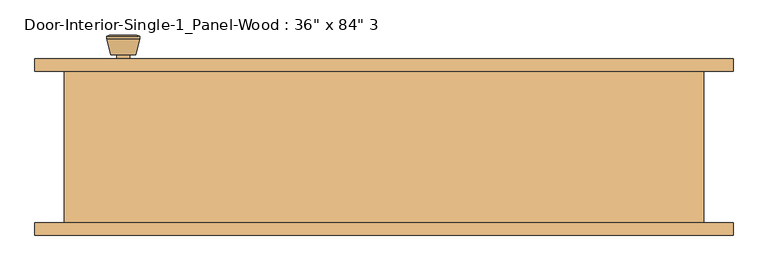
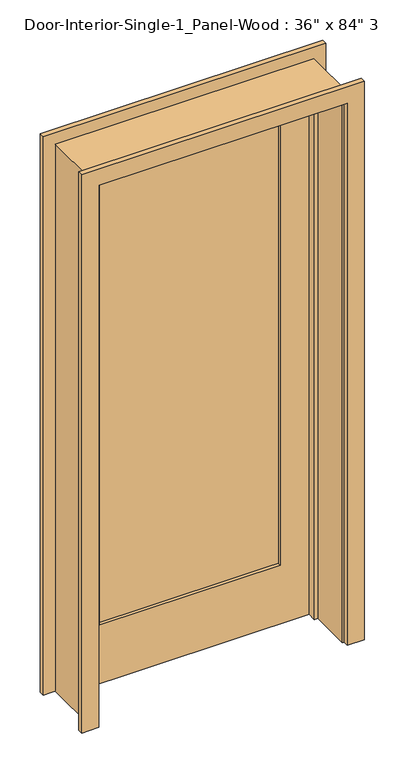
"""IFC4 building model written with IfcOpenShell, lengths in millimetres: door geometry."""

from ifc_helpers import new_model, si_unit, point, frame, frame_2d, origin, place, context, project, spatial, polyline, circle_curve, trimmed, segment, composite_curve, outline, extrude, faceted_brep, source, transform, mapped, element, save
from ifc_brep_helpers import plane_surface, cylinder_surface, revolved_surface, advanced_brep


def door_3b97b8e7(model_context):
    return source(origin(), model_context, "Body", "SolidModel", [
        advanced_brep(
        [(-393.7, 70.2, 914.4), (-383.7, 70.2, 914.4), (-403.7, 70.2, 914.4), (-373.2241324, 21.2, 914.4), (-393.7, 21.2, 914.4), (-414.1758676, 21.2, 914.4), (-368.7, 23.0278681, 914.4), (-418.7, 23.0278681, 914.4), (-368.7, 26.4915463, 914.4), (-418.7, 26.4915463, 914.4), (-375.063764, 51.2, 914.4), (-412.336236, 51.2, 914.4), (-383.7, 51.2, 914.4), (-403.7, 51.2, 914.4)],
        [
            (0, 1),
            (1, 2, circle_curve(frame((-393.7, 70.2, 914.4), z_axis=(0.0, 1.0, 0.0), x_axis=(-1.0, 0.0, 0.0)), 10.0)),
            (2, 0),
            (2, 1, circle_curve(frame((-393.7, 70.2, 914.4), z_axis=(0.0, 1.0, 0.0), x_axis=(-1.0, 0.0, 0.0)), 10.0)),
            (3, 4),
            (4, 5),
            (5, 3, circle_curve(frame((-393.7, 21.2, 914.4), z_axis=(0.0, -1.0, 0.0), x_axis=(-1.0, 0.0, 0.0)), 20.4758676)),
            (3, 5, circle_curve(frame((-393.7, 21.2, 914.4), z_axis=(0.0, -1.0, 0.0), x_axis=(-1.0, 0.0, 0.0)), 20.4758676)),
            (6, 3),
            (5, 7),
            (7, 6, circle_curve(frame((-393.7, 23.0278681, 914.4), z_axis=(0.0, -1.0, 0.0), x_axis=(-1.0, 0.0, 0.0)), 25.0)),
            (6, 7, circle_curve(frame((-393.7, 23.0278681, 914.4), z_axis=(0.0, -1.0, 0.0), x_axis=(-1.0, 0.0, 0.0)), 25.0)),
            (8, 6),
            (7, 9),
            (9, 8, circle_curve(frame((-393.7, 26.4915463, 914.4), z_axis=(0.0, -1.0, 0.0), x_axis=(-1.0, 0.0, 0.0)), 25.0)),
            (8, 9, circle_curve(frame((-393.7, 26.4915463, 914.4), z_axis=(0.0, -1.0, 0.0), x_axis=(-1.0, 0.0, 0.0)), 25.0)),
            (10, 8),
            (9, 11),
            (11, 10, circle_curve(frame((-393.7, 51.2, 914.4), z_axis=(0.0, -1.0, 0.0), x_axis=(-1.0, 0.0, 0.0)), 18.636236)),
            (10, 11, circle_curve(frame((-393.7, 51.2, 914.4), z_axis=(0.0, -1.0, 0.0), x_axis=(-1.0, 0.0, 0.0)), 18.636236)),
            (12, 10),
            (11, 13),
            (13, 12, circle_curve(frame((-393.7, 51.2, 914.4), z_axis=(0.0, -1.0, 0.0), x_axis=(-1.0, 0.0, 0.0)), 10.0)),
            (12, 13, circle_curve(frame((-393.7, 51.2, 914.4), z_axis=(0.0, -1.0, 0.0), x_axis=(-1.0, 0.0, 0.0)), 10.0)),
            (1, 12),
            (13, 2),
        ],
        [
            plane_surface(frame((-393.7, 70.2, 914.4), z_axis=(0.0, 1.0, 0.0), x_axis=(-1.0, 0.0, 0.0))),
            plane_surface(frame((-393.7, 21.2, 914.4), z_axis=(0.0, -1.0, 0.0), x_axis=(-1.0, 0.0, 0.0))),
            revolved_surface(polyline([(-414.1758676, 21.2, 914.4), (-418.7, 23.0278681, 914.4)]), (-393.7, 70.2, 914.4), (0.0, 1.0, 0.0)),
            cylinder_surface(frame((-393.7, 70.2, 914.4), z_axis=(0.0, 1.0, 0.0), x_axis=(-1.0, 0.0, 0.0)), 25.0),
            revolved_surface(polyline([(-418.7, 26.4915463, 914.4), (-412.336236, 51.2, 914.4)]), (-393.7, 70.2, 914.4), (0.0, 1.0, 0.0)),
            plane_surface(frame((-393.7, 51.2, 914.4), z_axis=(0.0, 1.0, 0.0), x_axis=(-1.0, 0.0, 0.0))),
            cylinder_surface(frame((-393.7, 70.2, 914.4), z_axis=(0.0, 1.0, 0.0), x_axis=(-1.0, 0.0, 0.0)), 10.0),
        ],
        [
            (0, [[1, 2, 3]]),
            (0, [[-3, 4, -1]]),
            (1, [[5, 6, 7]]),
            (1, [[-6, -5, 8]]),
            (2, [[9, -7, 10, 11]]),
            (2, [[-10, -8, -9, 12]]),
            (3, [[13, -11, 14, 15]]),
            (3, [[-14, -12, -13, 16]]),
            (4, [[17, -15, 18, 19]]),
            (4, [[-18, -16, -17, 20]]),
            (5, [[21, -19, 22, 23]]),
            (5, [[-22, -20, -21, 24]]),
            (6, [[25, -23, 26, -2]]),
            (6, [[-26, -24, -25, -4]]),
        ],
    ),
        extrude(outline(composite_curve([segment(trimmed(circle_curve(frame_2d((914.4, -393.7)), 30.0), [point((914.4, -423.7))], [point((914.4, -363.7))], False, "CARTESIAN"), True, "CONTINUOUS"), segment(trimmed(circle_curve(frame_2d((914.4, -393.7)), 30.0), [point((914.4, -363.7))], [point((914.4, -423.7))], False, "CARTESIAN"), True, "CONTINUOUS")], self_intersect=False)), frame((0.0, 70.2, 0.0), z_axis=(0.0, 1.0, 0.0), x_axis=(0.0, 0.0, 1.0)), (0.0, 0.0, 1.0), 6.0),
        advanced_brep(
        [(-393.7, 117.125, 914.4), (-403.7, 117.125, 914.4), (-383.7, 117.125, 914.4), (-373.2241324, 166.125, 914.4), (-414.1758676, 166.125, 914.4), (-393.7, 166.125, 914.4), (-368.7, 164.2971319, 914.4), (-418.7, 164.2971319, 914.4), (-368.7, 160.8334537, 914.4), (-418.7, 160.8334537, 914.4), (-375.063764, 136.125, 914.4), (-412.336236, 136.125, 914.4), (-383.7, 136.125, 914.4), (-403.7, 136.125, 914.4)],
        [
            (0, 1),
            (1, 2, circle_curve(frame((-393.7, 117.125, 914.4), z_axis=(0.0, -1.0, 0.0), x_axis=(-1.0, 0.0, 0.0)), 10.0)),
            (2, 0),
            (2, 1, circle_curve(frame((-393.7, 117.125, 914.4), z_axis=(0.0, -1.0, 0.0), x_axis=(-1.0, 0.0, 0.0)), 10.0)),
            (3, 4, circle_curve(frame((-393.7, 166.125, 914.4), z_axis=(0.0, 1.0, 0.0), x_axis=(-1.0, 0.0, 0.0)), 20.4758676)),
            (4, 5),
            (5, 3),
            (4, 3, circle_curve(frame((-393.7, 166.125, 914.4), z_axis=(0.0, 1.0, 0.0), x_axis=(-1.0, 0.0, 0.0)), 20.4758676)),
            (6, 7, circle_curve(frame((-393.7, 164.2971319, 914.4), z_axis=(0.0, 1.0, 0.0), x_axis=(-1.0, 0.0, 0.0)), 25.0)),
            (7, 4),
            (3, 6),
            (7, 6, circle_curve(frame((-393.7, 164.2971319, 914.4), z_axis=(0.0, 1.0, 0.0), x_axis=(-1.0, 0.0, 0.0)), 25.0)),
            (8, 9, circle_curve(frame((-393.7, 160.8334537, 914.4), z_axis=(0.0, 1.0, 0.0), x_axis=(-1.0, 0.0, 0.0)), 25.0)),
            (9, 7),
            (6, 8),
            (9, 8, circle_curve(frame((-393.7, 160.8334537, 914.4), z_axis=(0.0, 1.0, 0.0), x_axis=(-1.0, 0.0, 0.0)), 25.0)),
            (10, 11, circle_curve(frame((-393.7, 136.125, 914.4), z_axis=(0.0, 1.0, 0.0), x_axis=(-1.0, 0.0, 0.0)), 18.636236)),
            (11, 9),
            (8, 10),
            (11, 10, circle_curve(frame((-393.7, 136.125, 914.4), z_axis=(0.0, 1.0, 0.0), x_axis=(-1.0, 0.0, 0.0)), 18.636236)),
            (12, 13, circle_curve(frame((-393.7, 136.125, 914.4), z_axis=(0.0, 1.0, 0.0), x_axis=(-1.0, 0.0, 0.0)), 10.0)),
            (13, 11),
            (10, 12),
            (13, 12, circle_curve(frame((-393.7, 136.125, 914.4), z_axis=(0.0, 1.0, 0.0), x_axis=(-1.0, 0.0, 0.0)), 10.0)),
            (1, 13),
            (12, 2),
        ],
        [
            plane_surface(frame((-393.7, 117.125, 914.4), z_axis=(0.0, -1.0, 0.0), x_axis=(-1.0, 0.0, 0.0))),
            plane_surface(frame((-393.7, 166.125, 914.4), z_axis=(0.0, 1.0, 0.0), x_axis=(-1.0, 0.0, 0.0))),
            revolved_surface(polyline([(-414.1758676, 166.125, 914.4), (-418.7, 164.2971319, 914.4)]), (-393.7, 117.125, 914.4), (0.0, -1.0, 0.0)),
            cylinder_surface(frame((-393.7, 117.125, 914.4), z_axis=(0.0, -1.0, 0.0), x_axis=(-1.0, 0.0, 0.0)), 25.0),
            revolved_surface(polyline([(-418.7, 160.8334537, 914.4), (-412.336236, 136.125, 914.4)]), (-393.7, 117.125, 914.4), (0.0, -1.0, 0.0)),
            plane_surface(frame((-393.7, 136.125, 914.4), z_axis=(0.0, -1.0, 0.0), x_axis=(-1.0, 0.0, 0.0))),
            cylinder_surface(frame((-393.7, 117.125, 914.4), z_axis=(0.0, -1.0, 0.0), x_axis=(-1.0, 0.0, 0.0)), 10.0),
        ],
        [
            (0, [[1, 2, 3]]),
            (0, [[-3, 4, -1]]),
            (1, [[5, 6, 7]]),
            (1, [[8, -7, -6]]),
            (2, [[9, 10, -5, 11]]),
            (2, [[12, -11, -8, -10]]),
            (3, [[13, 14, -9, 15]]),
            (3, [[16, -15, -12, -14]]),
            (4, [[17, 18, -13, 19]]),
            (4, [[20, -19, -16, -18]]),
            (5, [[21, 22, -17, 23]]),
            (5, [[24, -23, -20, -22]]),
            (6, [[-2, 25, -21, 26]]),
            (6, [[-4, -26, -24, -25]]),
        ],
    ),
        extrude(outline(composite_curve([segment(trimmed(circle_curve(frame_2d((914.4, -393.7)), 30.0), [point((914.4, -423.7))], [point((914.4, -363.7))], False, "CARTESIAN"), True, "CONTINUOUS"), segment(trimmed(circle_curve(frame_2d((914.4, -393.7)), 30.0), [point((914.4, -363.7))], [point((914.4, -423.7))], False, "CARTESIAN"), True, "CONTINUOUS")], self_intersect=False)), frame((0.0, 111.125, 0.0), z_axis=(0.0, 1.0, 0.0), x_axis=(0.0, 0.0, 1.0)), (0.0, 0.0, 1.0), 6.0),
        faceted_brep([(482.6, 111.125, 0.0), (482.6, -117.475, 0.0), (457.2, -117.475, 0.0), (457.2, 41.275, 0.0), (444.5, 41.275, 0.0), (444.5, 76.2, 0.0), (457.2, 76.2, 0.0), (457.2, 111.125, 0.0), (482.6, 111.125, 2159.0), (482.6, -117.475, 2159.0), (-482.6, -117.475, 2159.0), (-482.6, -117.475, 0.0), (-457.2, -117.475, 0.0), (-457.2, -117.475, 2133.6), (457.2, -117.475, 2133.6), (457.2, 41.275, 2133.6), (-457.2, 41.275, 2133.6), (-457.2, 41.275, 0.0), (-444.5, 41.275, 0.0), (-444.5, 41.275, 2120.9), (444.5, 41.275, 2120.9), (444.5, 76.2, 2120.9), (-444.5, 76.2, 2120.9), (-444.5, 76.2, 0.0), (-457.2, 76.2, 0.0), (-457.2, 76.2, 2133.6), (457.2, 76.2, 2133.6), (457.2, 111.125, 2133.6), (-457.2, 111.125, 2133.6), (-457.2, 111.125, 0.0), (-482.6, 111.125, 0.0), (-482.6, 111.125, 2159.0)], [[[0, 1, 2, 3, 4, 5, 6, 7]], [[1, 0, 8, 9]], [[2, 1, 9, 10, 11, 12, 13, 14]], [[3, 2, 14, 15]], [[4, 3, 15, 16, 17, 18, 19, 20]], [[5, 4, 20, 21]], [[6, 5, 21, 22, 23, 24, 25, 26]], [[7, 6, 26, 27]], [[0, 7, 27, 28, 29, 30, 31, 8]], [[9, 8, 31, 10]], [[15, 14, 13, 16]], [[21, 20, 19, 22]], [[27, 26, 25, 28]], [[30, 29, 24, 23, 18, 17, 12, 11]], [[10, 31, 30, 11]], [[16, 13, 12, 17]], [[22, 19, 18, 23]], [[28, 25, 24, 29]]]),
        extrude(outline(polyline([(2133.6, -457.2), (0.0, -457.2), (0.0, 457.2), (2133.6, 457.2), (2133.6, -457.2)]), holes=[polyline([(2014.5375, -336.55), (2014.5375, 336.55), (231.775, 336.55), (231.775, -336.55), (2014.5375, -336.55)])]), frame((0.0, 76.2, 0.0), z_axis=(0.0, 1.0, 0.0), x_axis=(0.0, 0.0, 1.0)), (0.0, 0.0, 1.0), 34.925),
        extrude(outline(polyline([(336.55, 87.8416667), (-336.55, 87.8416667), (-336.55, 99.4833333), (336.55, 99.4833333), (336.55, 87.8416667)])), frame((0.0, 0.0, 231.775), z_axis=(0.0, 0.0, 1.0), x_axis=(1.0, 0.0, 0.0)), (0.0, 0.0, 1.0), 1782.7625),
        extrude(outline(polyline([(0.0, 463.55), (0.0, 527.05), (2203.45, 527.05), (2203.45, -527.05), (0.0, -527.05), (0.0, -463.55), (2139.95, -463.55), (2139.95, 463.55), (0.0, 463.55)])), frame((0.0, 111.125, 0.0), z_axis=(0.0, 1.0, 0.0), x_axis=(0.0, 0.0, 1.0)), (0.0, 0.0, 1.0), 19.05),
        extrude(outline(polyline([(0.0, 463.55), (0.0, 527.05), (2203.45, 527.05), (2203.45, -527.05), (0.0, -527.05), (0.0, -463.55), (2139.95, -463.55), (2139.95, 463.55), (0.0, 463.55)])), frame((0.0, -136.525, 0.0), z_axis=(0.0, 1.0, 0.0), x_axis=(0.0, 0.0, 1.0)), (0.0, 0.0, 1.0), 19.05),
    ])


if __name__ == "__main__":
    model = new_model("IFC4")
    model_context = context("Model", 3, world=origin())
    ifc_project = project(units=[si_unit("LENGTHUNIT", "METRE", prefix="MILLI")], contexts=[model_context])
    site = spatial("IfcSite", under=ifc_project)
    building = spatial("IfcBuilding", under=site)
    placement = place(None, origin())
    door_shape = door_3b97b8e7(model_context)
    element("IfcDoor", 1, ObjectType="Door-Interior-Single-1_Panel-Wood : 36\" x 84\" 3", at=placement, inside=building, context=model_context, shape_type="MappedRepresentation", body=[
        mapped(door_shape, transform((0.0, 0.0, 0.0), x_axis=(1.0, 0.0, 0.0), y_axis=(0.0, 1.0, 0.0), z_axis=(0.0, 0.0, 1.0))),
    ])
    save(model, "model.ifc")

# Revit data of these elements
# Type "Door-Interior-Single-1_Panel-Wood : 36\" x 84\" 3"
#   Type Mark = "10"
#   Assembly Code = "C1020300"
#   Analytic Construction = "Wooden"
#   Top Rail = 0' - 4 11/16"
#   Thickness = 0' - 1 3/8"
#   Thermal Resistance (R) = 2.5876 (h·ft²·°F)/BTU
#   Swing Angle [instance default] = 90.00°
#   Stiles = 0' - 4 3/4"
#   Rough Width = 3' - 2"
#   Rough Height = 7' - 1"
#   Height = 7' - 0"
#   Width = 3' - 0"
#   Heat Transfer Coefficient (U) = 0.3865 BTU/(h·ft²·°F)
#   Bottom Rail = 0' - 9 1/8"
#   Trim Material = door
#   Panel Material = door
#   Frame Material = door
#   Door Handle Material = Aluminum
#   Visual Light Transmittance = 0
#   Solar Heat Gain Coefficient = 0
#   Wall Closure = (empty or 0)
#   Function = (empty or 0)
# Element 1 (IfcDoor, "Door-Interior-Single-1_Panel-Wood : 36\" x 84\" 3")
#   Materials on its faces: "door", "Aluminum"
# Materials
#   "door": class "Generic", colour RGB 120 120 120, transparency 0, Cost = 0
#   "Aluminum": class "Metal", colour RGB 247 247 247, transparency 0, Description = "Aluminum 6061", Cost = 0
